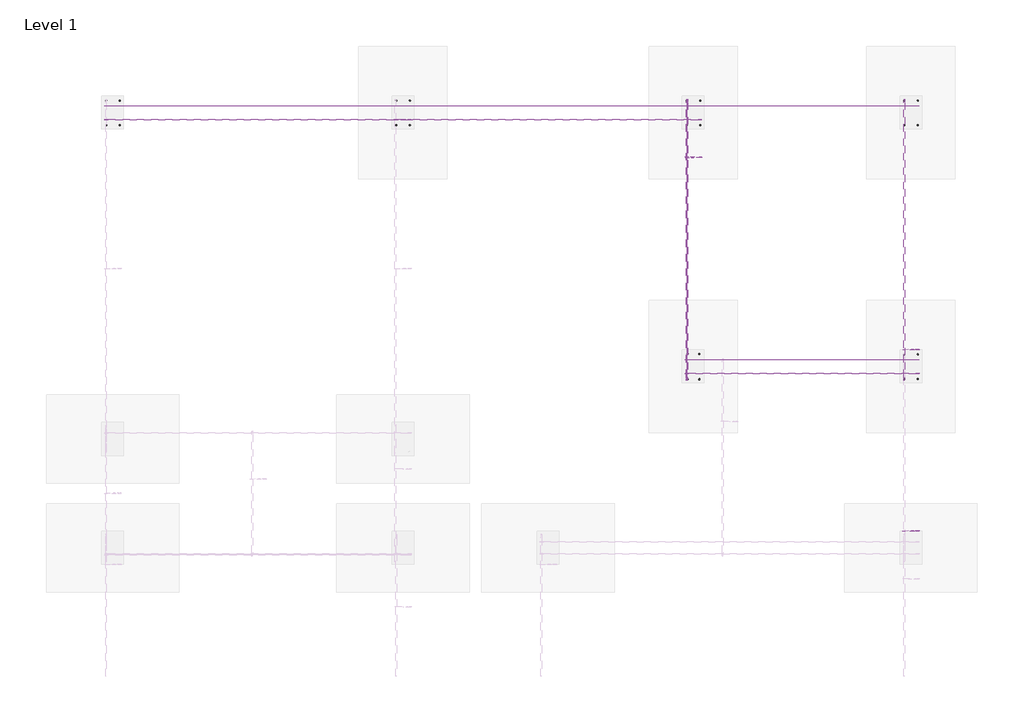
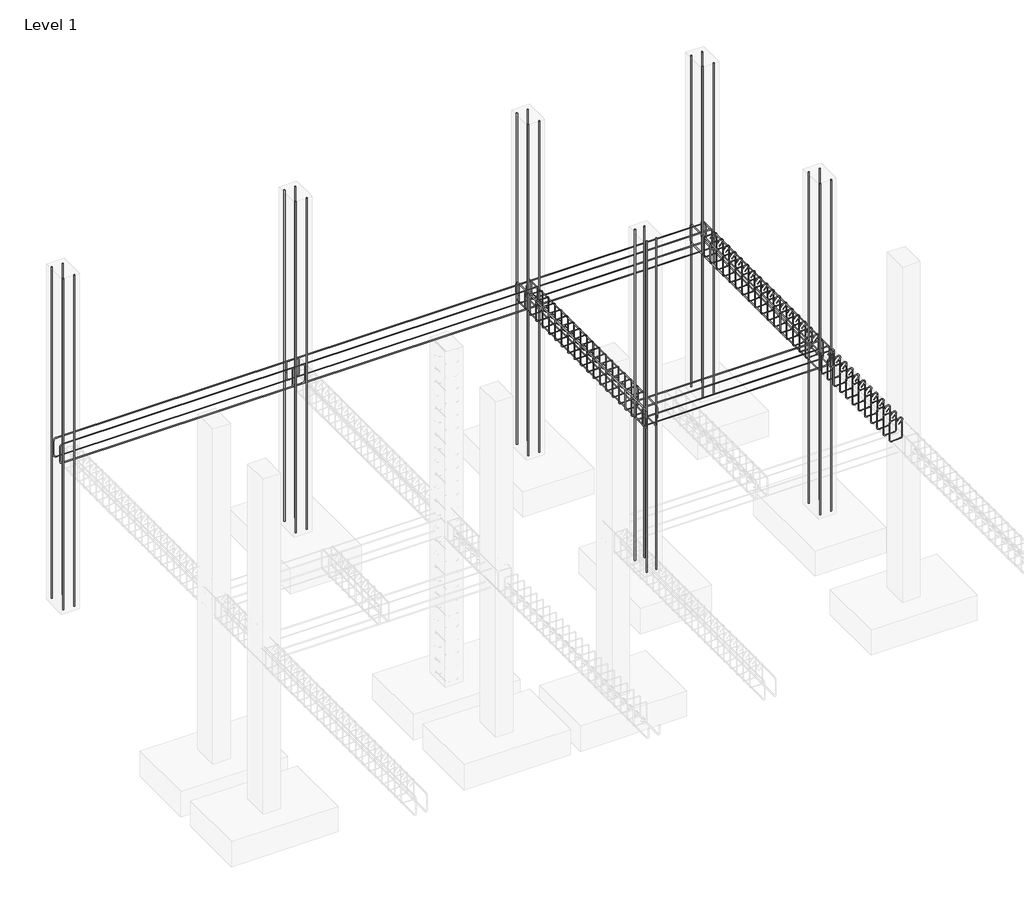
# One storey, part 5 of 5: 27 reinforcing bars.
"""IFC4 building model written with IfcOpenShell, lengths in millimetres."""

from ifc_helpers import new_model, si_unit, point, frame, origin, place, context, project, spatial, polyline, circle_curve, trimmed, segment, composite_curve, source, transform, mapped, element, save
from ifc_brep_helpers import swept_disk

model = new_model("IFC4")

# Units and contexts
model_context = context("Model", 3, world=origin())
ifc_project = project(units=[si_unit("LENGTHUNIT", "METRE", prefix="MILLI")], contexts=[model_context])

# Site, building, storey
site = spatial("IfcSite", under=ifc_project)
building = spatial("IfcBuilding", under=site)
storey = spatial("IfcBuildingStorey", under=building, Name="Level 1", Elevation=0.0)

# Reinforcing bars
placement = place(None, origin())
reinforcing_bar_shape = source(origin(), model_context, "Body", "SolidModel", [
    swept_disk(composite_curve([segment(polyline([(-15400.5504888, 8547.3557031, 38.1), (-15400.5504888, 8547.3557031, 6057.9)]), True, "CONTINUOUS")], self_intersect=False), 8.001),
])
element("IfcReinforcingBar", 1, at=placement, inside=storey, context=model_context, shape_type="MappedRepresentation", body=[
    mapped(reinforcing_bar_shape, transform((0.0, 0.0, 0.0), x_axis=(1.0, 0.0, 0.0), y_axis=(0.0, 1.0, 0.0), z_axis=(0.0, 0.0, 1.0))),
    mapped(reinforcing_bar_shape, transform((0.0, -339.0579018, 0.0), x_axis=(1.0, 0.0, 0.0), y_axis=(0.0, 1.0, 0.0), z_axis=(0.0, 0.0, 1.0))),
])
reinforcing_bar_2_shape = source(origin(), model_context, "Body", "SolidModel", [
    swept_disk(composite_curve([segment(polyline([(-15213.892587, 8547.3557031, 6057.9), (-15213.892587, 8547.3557031, 38.1)]), True, "CONTINUOUS")], self_intersect=False), 8.001),
])
element("IfcReinforcingBar", 2, at=placement, inside=storey, context=model_context, shape_type="MappedRepresentation", body=[
    mapped(reinforcing_bar_2_shape, transform((0.0, 0.0, 0.0), x_axis=(1.0, 0.0, 0.0), y_axis=(0.0, 1.0, 0.0), z_axis=(0.0, 0.0, 1.0))),
    mapped(reinforcing_bar_2_shape, transform((0.0, -339.0579018, 0.0), x_axis=(1.0, 0.0, 0.0), y_axis=(0.0, 1.0, 0.0), z_axis=(0.0, 0.0, 1.0))),
])
reinforcing_bar_3_shape = source(origin(), model_context, "Body", "SolidModel", [
    swept_disk(composite_curve([segment(polyline([(-11400.5504888, 8547.3557031, 38.1), (-11400.5504888, 8547.3557031, 6057.9)]), True, "CONTINUOUS")], self_intersect=False), 8.001),
])
element("IfcReinforcingBar", 3, at=placement, inside=storey, context=model_context, shape_type="MappedRepresentation", body=[
    mapped(reinforcing_bar_3_shape, transform((0.0, 0.0, 0.0), x_axis=(1.0, 0.0, 0.0), y_axis=(0.0, 1.0, 0.0), z_axis=(0.0, 0.0, 1.0))),
    mapped(reinforcing_bar_3_shape, transform((0.0, -339.0579018, 0.0), x_axis=(1.0, 0.0, 0.0), y_axis=(0.0, 1.0, 0.0), z_axis=(0.0, 0.0, 1.0))),
])
reinforcing_bar_4_shape = source(origin(), model_context, "Body", "SolidModel", [
    swept_disk(composite_curve([segment(polyline([(-11213.892587, 8547.3557031, 6057.9), (-11213.892587, 8547.3557031, 38.1)]), True, "CONTINUOUS")], self_intersect=False), 8.001),
])
element("IfcReinforcingBar", 4, at=placement, inside=storey, context=model_context, shape_type="MappedRepresentation", body=[
    mapped(reinforcing_bar_4_shape, transform((0.0, 0.0, 0.0), x_axis=(1.0, 0.0, 0.0), y_axis=(0.0, 1.0, 0.0), z_axis=(0.0, 0.0, 1.0))),
    mapped(reinforcing_bar_4_shape, transform((0.0, -339.0579018, 0.0), x_axis=(1.0, 0.0, 0.0), y_axis=(0.0, 1.0, 0.0), z_axis=(0.0, 0.0, 1.0))),
])
reinforcing_bar_5_shape = source(origin(), model_context, "Body", "SolidModel", [
    swept_disk(composite_curve([segment(polyline([(-7400.5504888, 8547.3557031, 38.1), (-7400.5504888, 8547.3557031, 6057.9)]), True, "CONTINUOUS")], self_intersect=False), 8.001),
])
element("IfcReinforcingBar", 5, at=placement, inside=storey, context=model_context, shape_type="MappedRepresentation", body=[
    mapped(reinforcing_bar_5_shape, transform((0.0, 0.0, 0.0), x_axis=(1.0, 0.0, 0.0), y_axis=(0.0, 1.0, 0.0), z_axis=(0.0, 0.0, 1.0))),
    mapped(reinforcing_bar_5_shape, transform((0.0, -339.0579018, 0.0), x_axis=(1.0, 0.0, 0.0), y_axis=(0.0, 1.0, 0.0), z_axis=(0.0, 0.0, 1.0))),
])
reinforcing_bar_6_shape = source(origin(), model_context, "Body", "SolidModel", [
    swept_disk(composite_curve([segment(polyline([(-7213.892587, 8547.3557031, 6057.9), (-7213.892587, 8547.3557031, 38.1)]), True, "CONTINUOUS")], self_intersect=False), 8.001),
])
element("IfcReinforcingBar", 6, at=placement, inside=storey, context=model_context, shape_type="MappedRepresentation", body=[
    mapped(reinforcing_bar_6_shape, transform((0.0, 0.0, 0.0), x_axis=(1.0, 0.0, 0.0), y_axis=(0.0, 1.0, 0.0), z_axis=(0.0, 0.0, 1.0))),
    mapped(reinforcing_bar_6_shape, transform((0.0, -339.0579018, 0.0), x_axis=(1.0, 0.0, 0.0), y_axis=(0.0, 1.0, 0.0), z_axis=(0.0, 0.0, 1.0))),
])
reinforcing_bar_7_shape = source(origin(), model_context, "Body", "SolidModel", [
    swept_disk(composite_curve([segment(polyline([(-4400.5504888, 8547.3557031, 38.1), (-4400.5504888, 8547.3557031, 6057.9)]), True, "CONTINUOUS")], self_intersect=False), 8.001),
])
element("IfcReinforcingBar", 7, at=placement, inside=storey, context=model_context, shape_type="MappedRepresentation", body=[
    mapped(reinforcing_bar_7_shape, transform((0.0, 0.0, 0.0), x_axis=(1.0, 0.0, 0.0), y_axis=(0.0, 1.0, 0.0), z_axis=(0.0, 0.0, 1.0))),
    mapped(reinforcing_bar_7_shape, transform((0.0, -339.0579018, 0.0), x_axis=(1.0, 0.0, 0.0), y_axis=(0.0, 1.0, 0.0), z_axis=(0.0, 0.0, 1.0))),
])
reinforcing_bar_8_shape = source(origin(), model_context, "Body", "SolidModel", [
    swept_disk(composite_curve([segment(polyline([(-4213.892587, 8547.3557031, 6057.9), (-4213.892587, 8547.3557031, 38.1)]), True, "CONTINUOUS")], self_intersect=False), 8.001),
])
element("IfcReinforcingBar", 8, at=placement, inside=storey, context=model_context, shape_type="MappedRepresentation", body=[
    mapped(reinforcing_bar_8_shape, transform((0.0, 0.0, 0.0), x_axis=(1.0, 0.0, 0.0), y_axis=(0.0, 1.0, 0.0), z_axis=(0.0, 0.0, 1.0))),
    mapped(reinforcing_bar_8_shape, transform((0.0, -339.0579018, 0.0), x_axis=(1.0, 0.0, 0.0), y_axis=(0.0, 1.0, 0.0), z_axis=(0.0, 0.0, 1.0))),
])
reinforcing_bar_9_shape = source(origin(), model_context, "Body", "SolidModel", [
    swept_disk(composite_curve([segment(polyline([(-11198.8905379, 8472.592544, 2844.9032081), (-11198.8905379, 8472.592544, 2692.5032081)]), True, "CONTINUOUS"), segment(trimmed(circle_curve(frame((-11242.9595379, 8472.592544, 2692.5032081), z_axis=(0.0, 1.0, 0.0), x_axis=(44.068999999999505, 0.0, 0.0)), 44.069), [point((-11198.8905379, 8472.592544, 2692.5032081))], [point((-11242.9595379, 8472.592544, 2648.4342081))], True, "CARTESIAN"), True, "CONTINUOUS"), segment(polyline([(-11242.9595379, 8472.592544, 2648.4342081), (-15371.4835379, 8472.592544, 2648.4342081)]), True, "CONTINUOUS"), segment(trimmed(circle_curve(frame((-15371.4835379, 8472.592544, 2692.5032081), z_axis=(0.0, 1.0, 0.0), x_axis=(0.0, 0.0, -44.06899999999996)), 44.069), [point((-15371.4835379, 8472.592544, 2648.4342081))], [point((-15415.5525379, 8472.592544, 2692.5032081))], True, "CARTESIAN"), True, "CONTINUOUS"), segment(polyline([(-15415.5525379, 8472.592544, 2692.5032081), (-15415.5525379, 8472.592544, 2844.9032081)]), True, "CONTINUOUS")], self_intersect=False), 5.969),
])
element("IfcReinforcingBar", 9, at=placement, inside=storey, context=model_context, shape_type="MappedRepresentation", body=[
    mapped(reinforcing_bar_9_shape, transform((0.0, 0.0, 0.0), x_axis=(1.0, 0.0, 0.0), y_axis=(0.0, 1.0, 0.0), z_axis=(0.0, 0.0, 1.0))),
    mapped(reinforcing_bar_9_shape, transform((0.0, -189.5315837, 0.0), x_axis=(1.0, 0.0, 0.0), y_axis=(0.0, 1.0, 0.0), z_axis=(0.0, 0.0, 1.0))),
])
reinforcing_bar_10_shape = source(origin(), model_context, "Body", "SolidModel", [
    swept_disk(composite_curve([segment(polyline([(-15415.5525379, 8472.592544, 2793.8967919), (-15415.5525379, 8472.592544, 2946.2967919)]), True, "CONTINUOUS"), segment(trimmed(circle_curve(frame((-15371.4835379, 8472.592544, 2946.2967919), z_axis=(0.0, 1.0, 0.0), x_axis=(-44.068999999999505, 0.0, 0.0)), 44.069), [point((-15415.5525379, 8472.592544, 2946.2967919))], [point((-15371.4835379, 8472.592544, 2990.3657919))], True, "CARTESIAN"), True, "CONTINUOUS"), segment(polyline([(-15371.4835379, 8472.592544, 2990.3657919), (-11242.9595379, 8472.592544, 2990.3657919)]), True, "CONTINUOUS"), segment(trimmed(circle_curve(frame((-11242.9595379, 8472.592544, 2946.2967919), z_axis=(0.0, 1.0, 0.0), x_axis=(0.0, 0.0, 44.069000000000415)), 44.069), [point((-11242.9595379, 8472.592544, 2990.3657919))], [point((-11198.8905379, 8472.592544, 2946.2967919))], True, "CARTESIAN"), True, "CONTINUOUS"), segment(polyline([(-11198.8905379, 8472.592544, 2946.2967919), (-11198.8905379, 8472.592544, 2793.8967919)]), True, "CONTINUOUS")], self_intersect=False), 5.969),
])
element("IfcReinforcingBar", 10, at=placement, inside=storey, context=model_context, shape_type="MappedRepresentation", body=[
    mapped(reinforcing_bar_10_shape, transform((0.0, 0.0, 0.0), x_axis=(1.0, 0.0, 0.0), y_axis=(0.0, 1.0, 0.0), z_axis=(0.0, 0.0, 1.0))),
    mapped(reinforcing_bar_10_shape, transform((0.0, -189.5315837, 0.0), x_axis=(1.0, 0.0, 0.0), y_axis=(0.0, 1.0, 0.0), z_axis=(0.0, 0.0, 1.0))),
])
reinforcing_bar_11_shape = source(origin(), model_context, "Body", "SolidModel", [
    swept_disk(composite_curve([segment(polyline([(-11415.5525379, 8472.592544, 2793.8967919), (-11415.5525379, 8472.592544, 2946.2967919)]), True, "CONTINUOUS"), segment(trimmed(circle_curve(frame((-11371.4835379, 8472.592544, 2946.2967919), z_axis=(0.0, 1.0, 0.0), x_axis=(-44.068999999999505, 0.0, 0.0)), 44.069), [point((-11415.5525379, 8472.592544, 2946.2967919))], [point((-11371.4835379, 8472.592544, 2990.3657919))], True, "CARTESIAN"), True, "CONTINUOUS"), segment(polyline([(-11371.4835379, 8472.592544, 2990.3657919), (-7242.9595379, 8472.592544, 2990.3657919)]), True, "CONTINUOUS"), segment(trimmed(circle_curve(frame((-7242.9595379, 8472.592544, 2946.2967919), z_axis=(0.0, 1.0, 0.0), x_axis=(0.0, 0.0, 44.069000000000415)), 44.069), [point((-7242.9595379, 8472.592544, 2990.3657919))], [point((-7198.8905379, 8472.592544, 2946.2967919))], True, "CARTESIAN"), True, "CONTINUOUS"), segment(polyline([(-7198.8905379, 8472.592544, 2946.2967919), (-7198.8905379, 8472.592544, 2793.8967919)]), True, "CONTINUOUS")], self_intersect=False), 5.969),
])
element("IfcReinforcingBar", 11, at=placement, inside=storey, context=model_context, shape_type="MappedRepresentation", body=[
    mapped(reinforcing_bar_11_shape, transform((0.0, 0.0, 0.0), x_axis=(1.0, 0.0, 0.0), y_axis=(0.0, 1.0, 0.0), z_axis=(0.0, 0.0, 1.0))),
    mapped(reinforcing_bar_11_shape, transform((0.0, -189.5315837, 0.0), x_axis=(1.0, 0.0, 0.0), y_axis=(0.0, 1.0, 0.0), z_axis=(0.0, 0.0, 1.0))),
])
reinforcing_bar_12_shape = source(origin(), model_context, "Body", "SolidModel", [
    swept_disk(composite_curve([segment(polyline([(-7198.8905379, 8472.592544, 2844.9032081), (-7198.8905379, 8472.592544, 2692.5032081)]), True, "CONTINUOUS"), segment(trimmed(circle_curve(frame((-7242.9595379, 8472.592544, 2692.5032081), z_axis=(0.0, 1.0, 0.0), x_axis=(44.069000000000415, 0.0, 0.0)), 44.069), [point((-7198.8905379, 8472.592544, 2692.5032081))], [point((-7242.9595379, 8472.592544, 2648.4342081))], True, "CARTESIAN"), True, "CONTINUOUS"), segment(polyline([(-7242.9595379, 8472.592544, 2648.4342081), (-11371.4835379, 8472.592544, 2648.4342081)]), True, "CONTINUOUS"), segment(trimmed(circle_curve(frame((-11371.4835379, 8472.592544, 2692.5032081), z_axis=(0.0, 1.0, 0.0), x_axis=(0.0, 0.0, -44.06899999999996)), 44.069), [point((-11371.4835379, 8472.592544, 2648.4342081))], [point((-11415.5525379, 8472.592544, 2692.5032081))], True, "CARTESIAN"), True, "CONTINUOUS"), segment(polyline([(-11415.5525379, 8472.592544, 2692.5032081), (-11415.5525379, 8472.592544, 2844.9032081)]), True, "CONTINUOUS")], self_intersect=False), 5.969),
])
element("IfcReinforcingBar", 12, at=placement, inside=storey, context=model_context, shape_type="MappedRepresentation", body=[
    mapped(reinforcing_bar_12_shape, transform((0.0, 0.0, 0.0), x_axis=(1.0, 0.0, 0.0), y_axis=(0.0, 1.0, 0.0), z_axis=(0.0, 0.0, 1.0))),
    mapped(reinforcing_bar_12_shape, transform((0.0, -189.5315837, 0.0), x_axis=(1.0, 0.0, 0.0), y_axis=(0.0, 1.0, 0.0), z_axis=(0.0, 0.0, 1.0))),
])
reinforcing_bar_13_shape = source(origin(), model_context, "Body", "SolidModel", [
    swept_disk(composite_curve([segment(polyline([(-7415.5525379, 8472.592544, 2793.8967919), (-7415.5525379, 8472.592544, 2946.2967919)]), True, "CONTINUOUS"), segment(trimmed(circle_curve(frame((-7371.4835379, 8472.592544, 2946.2967919), z_axis=(0.0, 1.0, 0.0), x_axis=(-44.069000000000415, 0.0, 0.0)), 44.069), [point((-7415.5525379, 8472.592544, 2946.2967919))], [point((-7371.4835379, 8472.592544, 2990.3657919))], True, "CARTESIAN"), True, "CONTINUOUS"), segment(polyline([(-7371.4835379, 8472.592544, 2990.3657919), (-4242.9595379, 8472.592544, 2990.3657919)]), True, "CONTINUOUS"), segment(trimmed(circle_curve(frame((-4242.9595379, 8472.592544, 2946.2967919), z_axis=(0.0, 1.0, 0.0), x_axis=(0.0, 0.0, 44.069000000000415)), 44.069), [point((-4242.9595379, 8472.592544, 2990.3657919))], [point((-4198.8905379, 8472.592544, 2946.2967919))], True, "CARTESIAN"), True, "CONTINUOUS"), segment(polyline([(-4198.8905379, 8472.592544, 2946.2967919), (-4198.8905379, 8472.592544, 2793.8967919)]), True, "CONTINUOUS")], self_intersect=False), 5.969),
])
element("IfcReinforcingBar", 13, at=placement, inside=storey, context=model_context, shape_type="MappedRepresentation", body=[
    mapped(reinforcing_bar_13_shape, transform((0.0, 0.0, 0.0), x_axis=(1.0, 0.0, 0.0), y_axis=(0.0, 1.0, 0.0), z_axis=(0.0, 0.0, 1.0))),
    mapped(reinforcing_bar_13_shape, transform((0.0, -189.5315837, 0.0), x_axis=(1.0, 0.0, 0.0), y_axis=(0.0, 1.0, 0.0), z_axis=(0.0, 0.0, 1.0))),
])
reinforcing_bar_14_shape = source(origin(), model_context, "Body", "SolidModel", [
    swept_disk(composite_curve([segment(polyline([(-4198.8905379, 8472.592544, 2844.9032081), (-4198.8905379, 8472.592544, 2692.5032081)]), True, "CONTINUOUS"), segment(trimmed(circle_curve(frame((-4242.9595379, 8472.592544, 2692.5032081), z_axis=(0.0, 1.0, 0.0), x_axis=(44.069000000000415, 0.0, 0.0)), 44.069), [point((-4198.8905379, 8472.592544, 2692.5032081))], [point((-4242.9595379, 8472.592544, 2648.4342081))], True, "CARTESIAN"), True, "CONTINUOUS"), segment(polyline([(-4242.9595379, 8472.592544, 2648.4342081), (-7371.4835379, 8472.592544, 2648.4342081)]), True, "CONTINUOUS"), segment(trimmed(circle_curve(frame((-7371.4835379, 8472.592544, 2692.5032081), z_axis=(0.0, 1.0, 0.0), x_axis=(0.0, 0.0, -44.06899999999996)), 44.069), [point((-7371.4835379, 8472.592544, 2648.4342081))], [point((-7415.5525379, 8472.592544, 2692.5032081))], True, "CARTESIAN"), True, "CONTINUOUS"), segment(polyline([(-7415.5525379, 8472.592544, 2692.5032081), (-7415.5525379, 8472.592544, 2844.9032081)]), True, "CONTINUOUS")], self_intersect=False), 5.969),
])
element("IfcReinforcingBar", 14, at=placement, inside=storey, context=model_context, shape_type="MappedRepresentation", body=[
    mapped(reinforcing_bar_14_shape, transform((0.0, 0.0, 0.0), x_axis=(1.0, 0.0, 0.0), y_axis=(0.0, 1.0, 0.0), z_axis=(0.0, 0.0, 1.0))),
    mapped(reinforcing_bar_14_shape, transform((0.0, -189.5315837, 0.0), x_axis=(1.0, 0.0, 0.0), y_axis=(0.0, 1.0, 0.0), z_axis=(0.0, 0.0, 1.0))),
])
reinforcing_bar_15_shape = source(origin(), model_context, "Body", "SolidModel", [
    swept_disk(composite_curve([segment(polyline([(-4212.455746, 8562.3577522, 2793.8967919), (-4212.455746, 8562.3577522, 2946.2967919)]), True, "CONTINUOUS"), segment(trimmed(circle_curve(frame((-4212.455746, 8518.2887522, 2946.2967919), z_axis=(1.0, 0.0, 0.0), x_axis=(0.0, 44.068999999999505, 0.0)), 44.069), [point((-4212.455746, 8562.3577522, 2946.2967919))], [point((-4212.455746, 8518.2887522, 2990.3657919))], True, "CARTESIAN"), True, "CONTINUOUS"), segment(polyline([(-4212.455746, 8518.2887522, 2990.3657919), (-4212.455746, 4737.3647522, 2990.3657919)]), True, "CONTINUOUS"), segment(trimmed(circle_curve(frame((-4212.455746, 4737.3647522, 2946.2967919), z_axis=(1.0, 0.0, 0.0), x_axis=(0.0, 0.0, 44.069000000000415)), 44.069), [point((-4212.455746, 4737.3647522, 2990.3657919))], [point((-4212.455746, 4693.2957522, 2946.2967919))], True, "CARTESIAN"), True, "CONTINUOUS"), segment(polyline([(-4212.455746, 4693.2957522, 2946.2967919), (-4212.455746, 4693.2957522, 2793.8967919)]), True, "CONTINUOUS")], self_intersect=False), 5.969),
])
element("IfcReinforcingBar", 15, at=placement, inside=storey, context=model_context, shape_type="MappedRepresentation", body=[
    mapped(reinforcing_bar_15_shape, transform((0.0, 0.0, 0.0), x_axis=(1.0, 0.0, 0.0), y_axis=(0.0, 1.0, 0.0), z_axis=(0.0, 0.0, 1.0))),
    mapped(reinforcing_bar_15_shape, transform((-189.5315837, 0.0, 0.0), x_axis=(1.0, 0.0, 0.0), y_axis=(0.0, 1.0, 0.0), z_axis=(0.0, 0.0, 1.0))),
])
reinforcing_bar_16_shape = source(origin(), model_context, "Body", "SolidModel", [
    swept_disk(composite_curve([segment(polyline([(-4212.455746, 4693.2957522, 2844.9032081), (-4212.455746, 4693.2957522, 2692.5032081)]), True, "CONTINUOUS"), segment(trimmed(circle_curve(frame((-4212.455746, 4737.3647522, 2692.5032081), z_axis=(1.0, 0.0, 0.0), x_axis=(0.0, -44.069000000000415, 0.0)), 44.069), [point((-4212.455746, 4693.2957522, 2692.5032081))], [point((-4212.455746, 4737.3647522, 2648.4342081))], True, "CARTESIAN"), True, "CONTINUOUS"), segment(polyline([(-4212.455746, 4737.3647522, 2648.4342081), (-4212.455746, 8518.2887522, 2648.4342081)]), True, "CONTINUOUS"), segment(trimmed(circle_curve(frame((-4212.455746, 8518.2887522, 2692.5032081), z_axis=(1.0, 0.0, 0.0), x_axis=(0.0, 0.0, -44.06899999999996)), 44.069), [point((-4212.455746, 8518.2887522, 2648.4342081))], [point((-4212.455746, 8562.3577522, 2692.5032081))], True, "CARTESIAN"), True, "CONTINUOUS"), segment(polyline([(-4212.455746, 8562.3577522, 2692.5032081), (-4212.455746, 8562.3577522, 2844.9032081)]), True, "CONTINUOUS")], self_intersect=False), 5.969),
])
element("IfcReinforcingBar", 16, at=placement, inside=storey, context=model_context, shape_type="MappedRepresentation", body=[
    mapped(reinforcing_bar_16_shape, transform((0.0, 0.0, 0.0), x_axis=(1.0, 0.0, 0.0), y_axis=(0.0, 1.0, 0.0), z_axis=(0.0, 0.0, 1.0))),
    mapped(reinforcing_bar_16_shape, transform((-189.5315837, 0.0, 0.0), x_axis=(1.0, 0.0, 0.0), y_axis=(0.0, 1.0, 0.0), z_axis=(0.0, 0.0, 1.0))),
])
reinforcing_bar_17_shape = source(origin(), model_context, "Body", "SolidModel", [
    swept_disk(composite_curve([segment(polyline([(-4213.892587, 5047.3557031, 38.1), (-4213.892587, 5047.3557031, 6057.9)]), True, "CONTINUOUS")], self_intersect=False), 8.001),
])
element("IfcReinforcingBar", 17, at=placement, inside=storey, context=model_context, shape_type="MappedRepresentation", body=[
    mapped(reinforcing_bar_17_shape, transform((0.0, 0.0, 0.0), x_axis=(1.0, 0.0, 0.0), y_axis=(0.0, 1.0, 0.0), z_axis=(0.0, 0.0, 1.0))),
    mapped(reinforcing_bar_17_shape, transform((-186.6579018, 0.0, 0.0), x_axis=(1.0, 0.0, 0.0), y_axis=(0.0, 1.0, 0.0), z_axis=(0.0, 0.0, 1.0))),
])
reinforcing_bar_18_shape = source(origin(), model_context, "Body", "SolidModel", [
    swept_disk(composite_curve([segment(polyline([(-4213.892587, 4708.2978013, 6057.9), (-4213.892587, 4708.2978013, 38.1)]), True, "CONTINUOUS")], self_intersect=False), 8.001),
])
element("IfcReinforcingBar", 18, at=placement, inside=storey, context=model_context, shape_type="MappedRepresentation", body=[
    mapped(reinforcing_bar_18_shape, transform((0.0, 0.0, 0.0), x_axis=(1.0, 0.0, 0.0), y_axis=(0.0, 1.0, 0.0), z_axis=(0.0, 0.0, 1.0))),
    mapped(reinforcing_bar_18_shape, transform((-186.6579018, 0.0, 0.0), x_axis=(1.0, 0.0, 0.0), y_axis=(0.0, 1.0, 0.0), z_axis=(0.0, 0.0, 1.0))),
])
reinforcing_bar_19_shape = source(origin(), model_context, "Body", "SolidModel", [
    swept_disk(composite_curve([segment(polyline([(-4260.3161447, 4645.2897522, 2901.0166099), (-4205.4511463, 4645.2897522, 2955.8816084)]), True, "CONTINUOUS"), segment(trimmed(circle_curve(frame((-4226.1955379, 4645.2897522, 2976.626), z_axis=(0.0, -1.0, 0.0), x_axis=(20.7443916000002, 0.0, -20.7443916000002)), 29.337), [point((-4205.4511463, 4645.2897522, 2955.8816084))], [point((-4226.1955379, 4645.2897522, 3005.963))], True, "CARTESIAN"), True, "CONTINUOUS"), segment(polyline([(-4226.1955379, 4645.2897522, 3005.963), (-4388.2475379, 4645.2897522, 3005.963)]), True, "CONTINUOUS"), segment(trimmed(circle_curve(frame((-4388.2475379, 4645.2897522, 2976.626), z_axis=(0.0, -1.0, 0.0), x_axis=(0.0, 0.0, 29.33699999999999)), 29.337), [point((-4388.2475379, 4645.2897522, 3005.963))], [point((-4417.5845379, 4645.2897522, 2976.626))], True, "CARTESIAN"), True, "CONTINUOUS"), segment(polyline([(-4417.5845379, 4645.2897522, 2976.626), (-4417.5845379, 4645.2897522, 2662.174)]), True, "CONTINUOUS"), segment(trimmed(circle_curve(frame((-4388.2661869, 4646.3356312, 2662.174), z_axis=(0.03565051078635044, -0.9993643184948482, 0.0), x_axis=(-29.318350999999893, -1.0458789999993314, 0.0)), 29.337), [point((-4417.5845379, 4645.2897522, 2662.174))], [point((-4388.2661869, 4646.3356312, 2632.837))], True, "CARTESIAN"), True, "CONTINUOUS"), segment(polyline([(-4388.2661869, 4646.3356312, 2632.837), (-4226.1768889, 4652.1178731, 2632.837)]), True, "CONTINUOUS"), segment(trimmed(circle_curve(frame((-4226.1768889, 4652.1178731, 2662.174), z_axis=(0.03565051078635044, -0.9993643184948482, 0.0), x_axis=(0.0, 0.0, -29.33699999999999)), 29.337), [point((-4226.1768889, 4652.1178731, 2632.837))], [point((-4196.8585379, 4653.1637522, 2662.174))], True, "CARTESIAN"), True, "CONTINUOUS"), segment(polyline([(-4196.8585379, 4653.1637522, 2662.174), (-4196.8585379, 4653.1637522, 2976.626)]), True, "CONTINUOUS"), segment(trimmed(circle_curve(frame((-4226.1955379, 4653.1637522, 2976.626), z_axis=(0.0, -1.0, 0.0), x_axis=(29.337000000000444, 0.0, 0.0)), 29.337), [point((-4196.8585379, 4653.1637522, 2976.626))], [point((-4246.9399295, 4653.1637522, 2997.3703916))], True, "CARTESIAN"), True, "CONTINUOUS"), segment(polyline([(-4246.9399295, 4653.1637522, 2997.3703916), (-4301.804928, 4653.1637522, 2942.5053932)]), True, "CONTINUOUS")], self_intersect=False), 3.937),
])
element("IfcReinforcingBar", 19, at=placement, inside=storey, context=model_context, shape_type="MappedRepresentation", body=[
    mapped(reinforcing_bar_19_shape, transform((0.0, 0.0, 0.0), x_axis=(1.0, 0.0, 0.0), y_axis=(0.0, 1.0, 0.0), z_axis=(0.0, 0.0, 1.0))),
    mapped(reinforcing_bar_19_shape, transform((0.0, -184.9932727, 0.0), x_axis=(1.0, 0.0, 0.0), y_axis=(0.0, 1.0, 0.0), z_axis=(0.0, 0.0, 1.0))),
    mapped(reinforcing_bar_19_shape, transform((0.0, -369.9865455, 0.0), x_axis=(1.0, 0.0, 0.0), y_axis=(0.0, 1.0, 0.0), z_axis=(0.0, 0.0, 1.0))),
    mapped(reinforcing_bar_19_shape, transform((0.0, -554.9798182, 0.0), x_axis=(1.0, 0.0, 0.0), y_axis=(0.0, 1.0, 0.0), z_axis=(0.0, 0.0, 1.0))),
    mapped(reinforcing_bar_19_shape, transform((0.0, -739.9730909, 0.0), x_axis=(1.0, 0.0, 0.0), y_axis=(0.0, 1.0, 0.0), z_axis=(0.0, 0.0, 1.0))),
    mapped(reinforcing_bar_19_shape, transform((0.0, -924.9663636, 0.0), x_axis=(1.0, 0.0, 0.0), y_axis=(0.0, 1.0, 0.0), z_axis=(0.0, 0.0, 1.0))),
    mapped(reinforcing_bar_19_shape, transform((0.0, -1109.9596364, 0.0), x_axis=(1.0, 0.0, 0.0), y_axis=(0.0, 1.0, 0.0), z_axis=(0.0, 0.0, 1.0))),
    mapped(reinforcing_bar_19_shape, transform((0.0, -1294.9529091, 0.0), x_axis=(1.0, 0.0, 0.0), y_axis=(0.0, 1.0, 0.0), z_axis=(0.0, 0.0, 1.0))),
    mapped(reinforcing_bar_19_shape, transform((0.0, -1479.9461818, 0.0), x_axis=(1.0, 0.0, 0.0), y_axis=(0.0, 1.0, 0.0), z_axis=(0.0, 0.0, 1.0))),
    mapped(reinforcing_bar_19_shape, transform((0.0, -1664.9394545, 0.0), x_axis=(1.0, 0.0, 0.0), y_axis=(0.0, 1.0, 0.0), z_axis=(0.0, 0.0, 1.0))),
    mapped(reinforcing_bar_19_shape, transform((0.0, -1849.9327273, 0.0), x_axis=(1.0, 0.0, 0.0), y_axis=(0.0, 1.0, 0.0), z_axis=(0.0, 0.0, 1.0))),
    mapped(reinforcing_bar_19_shape, transform((0.0, -2034.926, 0.0), x_axis=(1.0, 0.0, 0.0), y_axis=(0.0, 1.0, 0.0), z_axis=(0.0, 0.0, 1.0))),
])
reinforcing_bar_20_shape = source(origin(), model_context, "Body", "SolidModel", [
    swept_disk(composite_curve([segment(polyline([(-4260.3161447, 8145.2897522, 2901.0166099), (-4205.4511463, 8145.2897522, 2955.8816084)]), True, "CONTINUOUS"), segment(trimmed(circle_curve(frame((-4226.1955379, 8145.2897522, 2976.626), z_axis=(0.0, -1.0, 0.0), x_axis=(20.7443916000002, 0.0, -20.7443916000002)), 29.337), [point((-4205.4511463, 8145.2897522, 2955.8816084))], [point((-4226.1955379, 8145.2897522, 3005.963))], True, "CARTESIAN"), True, "CONTINUOUS"), segment(polyline([(-4226.1955379, 8145.2897522, 3005.963), (-4388.2475379, 8145.2897522, 3005.963)]), True, "CONTINUOUS"), segment(trimmed(circle_curve(frame((-4388.2475379, 8145.2897522, 2976.626), z_axis=(0.0, -1.0, 0.0), x_axis=(0.0, 0.0, 29.33699999999999)), 29.337), [point((-4388.2475379, 8145.2897522, 3005.963))], [point((-4417.5845379, 8145.2897522, 2976.626))], True, "CARTESIAN"), True, "CONTINUOUS"), segment(polyline([(-4417.5845379, 8145.2897522, 2976.626), (-4417.5845379, 8145.2897522, 2662.174)]), True, "CONTINUOUS"), segment(trimmed(circle_curve(frame((-4388.2661869, 8146.3356312, 2662.174), z_axis=(0.03565051078635027, -0.9993643184948483, 0.0), x_axis=(-29.318350999999893, -1.0458789999993314, 0.0)), 29.337), [point((-4417.5845379, 8145.2897522, 2662.174))], [point((-4388.2661869, 8146.3356312, 2632.837))], True, "CARTESIAN"), True, "CONTINUOUS"), segment(polyline([(-4388.2661869, 8146.3356312, 2632.837), (-4226.1768889, 8152.1178731, 2632.837)]), True, "CONTINUOUS"), segment(trimmed(circle_curve(frame((-4226.1768889, 8152.1178731, 2662.174), z_axis=(0.03565051078635027, -0.9993643184948483, 0.0), x_axis=(0.0, 0.0, -29.33699999999999)), 29.337), [point((-4226.1768889, 8152.1178731, 2632.837))], [point((-4196.8585379, 8153.1637522, 2662.174))], True, "CARTESIAN"), True, "CONTINUOUS"), segment(polyline([(-4196.8585379, 8153.1637522, 2662.174), (-4196.8585379, 8153.1637522, 2976.626)]), True, "CONTINUOUS"), segment(trimmed(circle_curve(frame((-4226.1955379, 8153.1637522, 2976.626), z_axis=(0.0, -1.0, 0.0), x_axis=(29.337000000000444, 0.0, 0.0)), 29.337), [point((-4196.8585379, 8153.1637522, 2976.626))], [point((-4246.9399295, 8153.1637522, 2997.3703916))], True, "CARTESIAN"), True, "CONTINUOUS"), segment(polyline([(-4246.9399295, 8153.1637522, 2997.3703916), (-4301.804928, 8153.1637522, 2942.5053932)]), True, "CONTINUOUS")], self_intersect=False), 3.937),
])
element("IfcReinforcingBar", 20, at=placement, inside=storey, context=model_context, shape_type="MappedRepresentation", body=[
    mapped(reinforcing_bar_20_shape, transform((0.0, 0.0, 0.0), x_axis=(1.0, 0.0, 0.0), y_axis=(0.0, 1.0, 0.0), z_axis=(0.0, 0.0, 1.0))),
    mapped(reinforcing_bar_20_shape, transform((0.0, -189.682875, 0.0), x_axis=(1.0, 0.0, 0.0), y_axis=(0.0, 1.0, 0.0), z_axis=(0.0, 0.0, 1.0))),
    mapped(reinforcing_bar_20_shape, transform((0.0, -379.36575, 0.0), x_axis=(1.0, 0.0, 0.0), y_axis=(0.0, 1.0, 0.0), z_axis=(0.0, 0.0, 1.0))),
    mapped(reinforcing_bar_20_shape, transform((0.0, -569.048625, 0.0), x_axis=(1.0, 0.0, 0.0), y_axis=(0.0, 1.0, 0.0), z_axis=(0.0, 0.0, 1.0))),
    mapped(reinforcing_bar_20_shape, transform((0.0, -758.7315, 0.0), x_axis=(1.0, 0.0, 0.0), y_axis=(0.0, 1.0, 0.0), z_axis=(0.0, 0.0, 1.0))),
    mapped(reinforcing_bar_20_shape, transform((0.0, -948.414375, 0.0), x_axis=(1.0, 0.0, 0.0), y_axis=(0.0, 1.0, 0.0), z_axis=(0.0, 0.0, 1.0))),
    mapped(reinforcing_bar_20_shape, transform((0.0, -1138.09725, 0.0), x_axis=(1.0, 0.0, 0.0), y_axis=(0.0, 1.0, 0.0), z_axis=(0.0, 0.0, 1.0))),
    mapped(reinforcing_bar_20_shape, transform((0.0, -1327.780125, 0.0), x_axis=(1.0, 0.0, 0.0), y_axis=(0.0, 1.0, 0.0), z_axis=(0.0, 0.0, 1.0))),
    mapped(reinforcing_bar_20_shape, transform((0.0, -1517.463, 0.0), x_axis=(1.0, 0.0, 0.0), y_axis=(0.0, 1.0, 0.0), z_axis=(0.0, 0.0, 1.0))),
    mapped(reinforcing_bar_20_shape, transform((0.0, -1707.145875, 0.0), x_axis=(1.0, 0.0, 0.0), y_axis=(0.0, 1.0, 0.0), z_axis=(0.0, 0.0, 1.0))),
    mapped(reinforcing_bar_20_shape, transform((0.0, -1896.82875, 0.0), x_axis=(1.0, 0.0, 0.0), y_axis=(0.0, 1.0, 0.0), z_axis=(0.0, 0.0, 1.0))),
    mapped(reinforcing_bar_20_shape, transform((0.0, -2086.511625, 0.0), x_axis=(1.0, 0.0, 0.0), y_axis=(0.0, 1.0, 0.0), z_axis=(0.0, 0.0, 1.0))),
    mapped(reinforcing_bar_20_shape, transform((0.0, -2276.1945, 0.0), x_axis=(1.0, 0.0, 0.0), y_axis=(0.0, 1.0, 0.0), z_axis=(0.0, 0.0, 1.0))),
    mapped(reinforcing_bar_20_shape, transform((0.0, -2465.877375, 0.0), x_axis=(1.0, 0.0, 0.0), y_axis=(0.0, 1.0, 0.0), z_axis=(0.0, 0.0, 1.0))),
    mapped(reinforcing_bar_20_shape, transform((0.0, -2655.56025, 0.0), x_axis=(1.0, 0.0, 0.0), y_axis=(0.0, 1.0, 0.0), z_axis=(0.0, 0.0, 1.0))),
    mapped(reinforcing_bar_20_shape, transform((0.0, -2845.243125, 0.0), x_axis=(1.0, 0.0, 0.0), y_axis=(0.0, 1.0, 0.0), z_axis=(0.0, 0.0, 1.0))),
    mapped(reinforcing_bar_20_shape, transform((0.0, -3034.926, 0.0), x_axis=(1.0, 0.0, 0.0), y_axis=(0.0, 1.0, 0.0), z_axis=(0.0, 0.0, 1.0))),
])
reinforcing_bar_21_shape = source(origin(), model_context, "Body", "SolidModel", [
    swept_disk(composite_curve([segment(polyline([(-7354.1269311, 5110.3637522, 2901.0166099), (-7408.9919295, 5110.3637522, 2955.8816084)]), True, "CONTINUOUS"), segment(trimmed(circle_curve(frame((-7388.2475379, 5110.3637522, 2976.626), z_axis=(0.0, 1.0, 0.0), x_axis=(-20.7443916000002, 0.0, -20.7443916000002)), 29.337), [point((-7408.9919295, 5110.3637522, 2955.8816084))], [point((-7388.2475379, 5110.3637522, 3005.963))], True, "CARTESIAN"), True, "CONTINUOUS"), segment(polyline([(-7388.2475379, 5110.3637522, 3005.963), (-7226.1955379, 5110.3637522, 3005.963)]), True, "CONTINUOUS"), segment(trimmed(circle_curve(frame((-7226.1955379, 5110.3637522, 2976.626), z_axis=(0.0, 1.0, 0.0), x_axis=(0.0, 0.0, 29.33699999999999)), 29.337), [point((-7226.1955379, 5110.3637522, 3005.963))], [point((-7196.8585379, 5110.3637522, 2976.626))], True, "CARTESIAN"), True, "CONTINUOUS"), segment(polyline([(-7196.8585379, 5110.3637522, 2976.626), (-7196.8585379, 5110.3637522, 2662.174)]), True, "CONTINUOUS"), segment(trimmed(circle_curve(frame((-7226.1768889, 5109.3178731, 2662.174), z_axis=(-0.03565051078635081, 0.9993643184948481, 0.0), x_axis=(29.318351000000803, 1.0458791000000929, 0.0)), 29.337), [point((-7196.8585379, 5110.3637522, 2662.174))], [point((-7226.1768889, 5109.3178731, 2632.837))], True, "CARTESIAN"), True, "CONTINUOUS"), segment(polyline([(-7226.1768889, 5109.3178731, 2632.837), (-7388.2661869, 5103.5356312, 2632.837)]), True, "CONTINUOUS"), segment(trimmed(circle_curve(frame((-7388.2661869, 5103.5356312, 2662.174), z_axis=(-0.03565051078635081, 0.9993643184948481, 0.0), x_axis=(0.0, 0.0, -29.33699999999999)), 29.337), [point((-7388.2661869, 5103.5356312, 2632.837))], [point((-7417.5845379, 5102.4897522, 2662.174))], True, "CARTESIAN"), True, "CONTINUOUS"), segment(polyline([(-7417.5845379, 5102.4897522, 2662.174), (-7417.5845379, 5102.4897522, 2976.626)]), True, "CONTINUOUS"), segment(trimmed(circle_curve(frame((-7388.2475379, 5102.4897522, 2976.626), z_axis=(0.0, 1.0, 0.0), x_axis=(-29.337000000000444, 0.0, 0.0)), 29.337), [point((-7417.5845379, 5102.4897522, 2976.626))], [point((-7367.5031463, 5102.4897522, 2997.3703916))], True, "CARTESIAN"), True, "CONTINUOUS"), segment(polyline([(-7367.5031463, 5102.4897522, 2997.3703916), (-7312.6381478, 5102.4897522, 2942.5053932)]), True, "CONTINUOUS")], self_intersect=False), 3.937),
])
element("IfcReinforcingBar", 21, at=placement, inside=storey, context=model_context, shape_type="MappedRepresentation", body=[
    mapped(reinforcing_bar_21_shape, transform((0.0, 0.0, 0.0), x_axis=(1.0, 0.0, 0.0), y_axis=(0.0, 1.0, 0.0), z_axis=(0.0, 0.0, 1.0))),
    mapped(reinforcing_bar_21_shape, transform((0.0, 189.682875, 0.0), x_axis=(1.0, 0.0, 0.0), y_axis=(0.0, 1.0, 0.0), z_axis=(0.0, 0.0, 1.0))),
    mapped(reinforcing_bar_21_shape, transform((0.0, 379.36575, 0.0), x_axis=(1.0, 0.0, 0.0), y_axis=(0.0, 1.0, 0.0), z_axis=(0.0, 0.0, 1.0))),
    mapped(reinforcing_bar_21_shape, transform((0.0, 569.048625, 0.0), x_axis=(1.0, 0.0, 0.0), y_axis=(0.0, 1.0, 0.0), z_axis=(0.0, 0.0, 1.0))),
    mapped(reinforcing_bar_21_shape, transform((0.0, 758.7315, 0.0), x_axis=(1.0, 0.0, 0.0), y_axis=(0.0, 1.0, 0.0), z_axis=(0.0, 0.0, 1.0))),
    mapped(reinforcing_bar_21_shape, transform((0.0, 948.414375, 0.0), x_axis=(1.0, 0.0, 0.0), y_axis=(0.0, 1.0, 0.0), z_axis=(0.0, 0.0, 1.0))),
    mapped(reinforcing_bar_21_shape, transform((0.0, 1138.09725, 0.0), x_axis=(1.0, 0.0, 0.0), y_axis=(0.0, 1.0, 0.0), z_axis=(0.0, 0.0, 1.0))),
    mapped(reinforcing_bar_21_shape, transform((0.0, 1327.780125, 0.0), x_axis=(1.0, 0.0, 0.0), y_axis=(0.0, 1.0, 0.0), z_axis=(0.0, 0.0, 1.0))),
    mapped(reinforcing_bar_21_shape, transform((0.0, 1517.463, 0.0), x_axis=(1.0, 0.0, 0.0), y_axis=(0.0, 1.0, 0.0), z_axis=(0.0, 0.0, 1.0))),
    mapped(reinforcing_bar_21_shape, transform((0.0, 1707.145875, 0.0), x_axis=(1.0, 0.0, 0.0), y_axis=(0.0, 1.0, 0.0), z_axis=(0.0, 0.0, 1.0))),
    mapped(reinforcing_bar_21_shape, transform((0.0, 1896.82875, 0.0), x_axis=(1.0, 0.0, 0.0), y_axis=(0.0, 1.0, 0.0), z_axis=(0.0, 0.0, 1.0))),
    mapped(reinforcing_bar_21_shape, transform((0.0, 2086.511625, 0.0), x_axis=(1.0, 0.0, 0.0), y_axis=(0.0, 1.0, 0.0), z_axis=(0.0, 0.0, 1.0))),
    mapped(reinforcing_bar_21_shape, transform((0.0, 2276.1945, 0.0), x_axis=(1.0, 0.0, 0.0), y_axis=(0.0, 1.0, 0.0), z_axis=(0.0, 0.0, 1.0))),
    mapped(reinforcing_bar_21_shape, transform((0.0, 2465.877375, 0.0), x_axis=(1.0, 0.0, 0.0), y_axis=(0.0, 1.0, 0.0), z_axis=(0.0, 0.0, 1.0))),
    mapped(reinforcing_bar_21_shape, transform((0.0, 2655.56025, 0.0), x_axis=(1.0, 0.0, 0.0), y_axis=(0.0, 1.0, 0.0), z_axis=(0.0, 0.0, 1.0))),
    mapped(reinforcing_bar_21_shape, transform((0.0, 2845.243125, 0.0), x_axis=(1.0, 0.0, 0.0), y_axis=(0.0, 1.0, 0.0), z_axis=(0.0, 0.0, 1.0))),
    mapped(reinforcing_bar_21_shape, transform((0.0, 3034.926, 0.0), x_axis=(1.0, 0.0, 0.0), y_axis=(0.0, 1.0, 0.0), z_axis=(0.0, 0.0, 1.0))),
])
reinforcing_bar_22_shape = source(origin(), model_context, "Body", "SolidModel", [
    swept_disk(composite_curve([segment(polyline([(-7401.9873298, 4693.2957522, 2793.8967919), (-7401.9873298, 4693.2957522, 2946.2967919)]), True, "CONTINUOUS"), segment(trimmed(circle_curve(frame((-7401.9873298, 4737.3647522, 2946.2967919), z_axis=(-1.0, 0.0, 0.0), x_axis=(0.0, -44.069000000000415, 0.0)), 44.069), [point((-7401.9873298, 4693.2957522, 2946.2967919))], [point((-7401.9873298, 4737.3647522, 2990.3657919))], True, "CARTESIAN"), True, "CONTINUOUS"), segment(polyline([(-7401.9873298, 4737.3647522, 2990.3657919), (-7401.9873298, 8518.2887522, 2990.3657919)]), True, "CONTINUOUS"), segment(trimmed(circle_curve(frame((-7401.9873298, 8518.2887522, 2946.2967919), z_axis=(-1.0, 0.0, 0.0), x_axis=(0.0, 0.0, 44.069000000000415)), 44.069), [point((-7401.9873298, 8518.2887522, 2990.3657919))], [point((-7401.9873298, 8562.3577522, 2946.2967919))], True, "CARTESIAN"), True, "CONTINUOUS"), segment(polyline([(-7401.9873298, 8562.3577522, 2946.2967919), (-7401.9873298, 8562.3577522, 2793.8967919)]), True, "CONTINUOUS")], self_intersect=False), 5.969),
])
element("IfcReinforcingBar", 22, at=placement, inside=storey, context=model_context, shape_type="MappedRepresentation", body=[
    mapped(reinforcing_bar_22_shape, transform((0.0, 0.0, 0.0), x_axis=(1.0, 0.0, 0.0), y_axis=(0.0, 1.0, 0.0), z_axis=(0.0, 0.0, 1.0))),
    mapped(reinforcing_bar_22_shape, transform((189.5315837, 0.0, 0.0), x_axis=(1.0, 0.0, 0.0), y_axis=(0.0, 1.0, 0.0), z_axis=(0.0, 0.0, 1.0))),
])
reinforcing_bar_23_shape = source(origin(), model_context, "Body", "SolidModel", [
    swept_disk(composite_curve([segment(polyline([(-7226.1955379, 8562.3577522, 2839.212), (-7226.1955379, 8562.3577522, 2686.812)]), True, "CONTINUOUS"), segment(trimmed(circle_curve(frame((-7226.1955379, 8518.2887522, 2686.812), z_axis=(-1.0, 0.0, 0.0), x_axis=(0.0, 44.068999999999505, 0.0)), 44.069), [point((-7226.1955379, 8562.3577522, 2686.812))], [point((-7226.1955379, 8518.2887522, 2642.743))], True, "CARTESIAN"), True, "CONTINUOUS"), segment(polyline([(-7226.1955379, 8518.2887522, 2642.743), (-7226.1955379, 4737.3647522, 2642.743)]), True, "CONTINUOUS"), segment(trimmed(circle_curve(frame((-7226.1955379, 4737.3647522, 2686.812), z_axis=(-1.0, 0.0, 0.0), x_axis=(0.0, 0.0, -44.06899999999996)), 44.069), [point((-7226.1955379, 4737.3647522, 2642.743))], [point((-7226.1955379, 4693.2957522, 2686.812))], True, "CARTESIAN"), True, "CONTINUOUS"), segment(polyline([(-7226.1955379, 4693.2957522, 2686.812), (-7226.1955379, 4693.2957522, 2839.212)]), True, "CONTINUOUS")], self_intersect=False), 5.969),
])
element("IfcReinforcingBar", 23, at=placement, inside=storey, context=model_context, shape_type="MappedRepresentation", body=[
    mapped(reinforcing_bar_23_shape, transform((0.0, 0.0, 0.0), x_axis=(1.0, 0.0, 0.0), y_axis=(0.0, 1.0, 0.0), z_axis=(0.0, 0.0, 1.0))),
    mapped(reinforcing_bar_23_shape, transform((-162.052, 0.0, 0.0), x_axis=(1.0, 0.0, 0.0), y_axis=(0.0, 1.0, 0.0), z_axis=(0.0, 0.0, 1.0))),
])
reinforcing_bar_24_shape = source(origin(), model_context, "Body", "SolidModel", [
    swept_disk(composite_curve([segment(polyline([(-7226.1955379, 4703.2017522, 38.1), (-7226.1955379, 4703.2017522, 6057.9)]), True, "CONTINUOUS")], self_intersect=False), 8.001),
])
element("IfcReinforcingBar", 24, at=placement, inside=storey, context=model_context, shape_type="MappedRepresentation", body=[
    mapped(reinforcing_bar_24_shape, transform((0.0, 0.0, 0.0), x_axis=(1.0, 0.0, 0.0), y_axis=(0.0, 1.0, 0.0), z_axis=(0.0, 0.0, 1.0))),
    mapped(reinforcing_bar_24_shape, transform((-162.052, 0.0, 0.0), x_axis=(1.0, 0.0, 0.0), y_axis=(0.0, 1.0, 0.0), z_axis=(0.0, 0.0, 1.0))),
])
reinforcing_bar_25_shape = source(origin(), model_context, "Body", "SolidModel", [
    swept_disk(composite_curve([segment(polyline([(-7388.2475379, 5052.4517522, 6057.9), (-7388.2475379, 5052.4517522, 38.1)]), True, "CONTINUOUS")], self_intersect=False), 8.001),
])
element("IfcReinforcingBar", 25, at=placement, inside=storey, context=model_context, shape_type="MappedRepresentation", body=[
    mapped(reinforcing_bar_25_shape, transform((0.0, 0.0, 0.0), x_axis=(1.0, 0.0, 0.0), y_axis=(0.0, 1.0, 0.0), z_axis=(0.0, 0.0, 1.0))),
    mapped(reinforcing_bar_25_shape, transform((162.052, 0.0, 0.0), x_axis=(1.0, 0.0, 0.0), y_axis=(0.0, 1.0, 0.0), z_axis=(0.0, 0.0, 1.0))),
])
reinforcing_bar_26_shape = source(origin(), model_context, "Body", "SolidModel", [
    swept_disk(composite_curve([segment(polyline([(-4198.8905379, 4783.0609603, 2793.8967919), (-4198.8905379, 4783.0609603, 2946.2967919)]), True, "CONTINUOUS"), segment(trimmed(circle_curve(frame((-4242.9595379, 4783.0609603, 2946.2967919), z_axis=(0.0, -1.0, 0.0), x_axis=(44.069000000000415, 0.0, 0.0)), 44.069), [point((-4198.8905379, 4783.0609603, 2946.2967919))], [point((-4242.9595379, 4783.0609603, 2990.3657919))], True, "CARTESIAN"), True, "CONTINUOUS"), segment(polyline([(-4242.9595379, 4783.0609603, 2990.3657919), (-7371.4835379, 4783.0609603, 2990.3657919)]), True, "CONTINUOUS"), segment(trimmed(circle_curve(frame((-7371.4835379, 4783.0609603, 2946.2967919), z_axis=(0.0, -1.0, 0.0), x_axis=(0.0, 0.0, 44.069000000000415)), 44.069), [point((-7371.4835379, 4783.0609603, 2990.3657919))], [point((-7415.5525379, 4783.0609603, 2946.2967919))], True, "CARTESIAN"), True, "CONTINUOUS"), segment(polyline([(-7415.5525379, 4783.0609603, 2946.2967919), (-7415.5525379, 4783.0609603, 2793.8967919)]), True, "CONTINUOUS")], self_intersect=False), 5.969),
])
element("IfcReinforcingBar", 26, at=placement, inside=storey, context=model_context, shape_type="MappedRepresentation", body=[
    mapped(reinforcing_bar_26_shape, transform((0.0, 0.0, 0.0), x_axis=(1.0, 0.0, 0.0), y_axis=(0.0, 1.0, 0.0), z_axis=(0.0, 0.0, 1.0))),
    mapped(reinforcing_bar_26_shape, transform((0.0, 189.5315837, 0.0), x_axis=(1.0, 0.0, 0.0), y_axis=(0.0, 1.0, 0.0), z_axis=(0.0, 0.0, 1.0))),
])
reinforcing_bar_27_shape = source(origin(), model_context, "Body", "SolidModel", [
    swept_disk(composite_curve([segment(polyline([(-7415.5525379, 4783.0609603, 2844.9032081), (-7415.5525379, 4783.0609603, 2692.5032081)]), True, "CONTINUOUS"), segment(trimmed(circle_curve(frame((-7371.4835379, 4783.0609603, 2692.5032081), z_axis=(0.0, -1.0, 0.0), x_axis=(-44.069000000000415, 0.0, 0.0)), 44.069), [point((-7415.5525379, 4783.0609603, 2692.5032081))], [point((-7371.4835379, 4783.0609603, 2648.4342081))], True, "CARTESIAN"), True, "CONTINUOUS"), segment(polyline([(-7371.4835379, 4783.0609603, 2648.4342081), (-4242.9595379, 4783.0609603, 2648.4342081)]), True, "CONTINUOUS"), segment(trimmed(circle_curve(frame((-4242.9595379, 4783.0609603, 2692.5032081), z_axis=(0.0, -1.0, 0.0), x_axis=(0.0, 0.0, -44.06899999999996)), 44.069), [point((-4242.9595379, 4783.0609603, 2648.4342081))], [point((-4198.8905379, 4783.0609603, 2692.5032081))], True, "CARTESIAN"), True, "CONTINUOUS"), segment(polyline([(-4198.8905379, 4783.0609603, 2692.5032081), (-4198.8905379, 4783.0609603, 2844.9032081)]), True, "CONTINUOUS")], self_intersect=False), 5.969),
])
element("IfcReinforcingBar", 27, at=placement, inside=storey, context=model_context, shape_type="MappedRepresentation", body=[
    mapped(reinforcing_bar_27_shape, transform((0.0, 0.0, 0.0), x_axis=(1.0, 0.0, 0.0), y_axis=(0.0, 1.0, 0.0), z_axis=(0.0, 0.0, 1.0))),
    mapped(reinforcing_bar_27_shape, transform((0.0, 189.5315837, 0.0), x_axis=(1.0, 0.0, 0.0), y_axis=(0.0, 1.0, 0.0), z_axis=(0.0, 0.0, 1.0))),
])

save(model, "model.ifc")

# Revit data of these elements
# Elements 1, 2, 3, 4, 5, 6, 7, 8, 9, 10, 11, 12, 13, 14, 15, 16, 17, 18, 19, 20, 21, 22, 23, 24, 25, 26, 27 (IfcReinforcingBar)
#   Phase Created = New Construction
